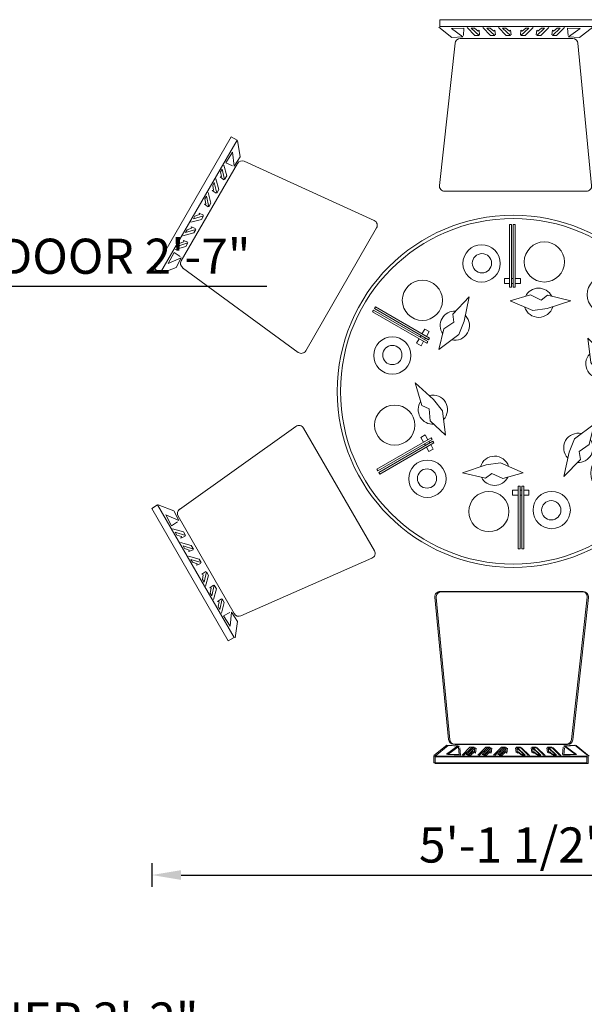
# Model space of a CAD drawing. Units: inches. Extents: x 1961 to 3038, y 800 to 1438.
# Tile 5 of 13: x 2755 to 2803, y 1058 to 1143. Entities that reach past the tile are written whole.
import ezdxf

# ---------------------------------------------------------------- set-up
doc = ezdxf.new("R2010")
doc.units = ezdxf.units.IN
doc.layers.add('A-ANNO-DIMS', color=2, linetype='Continuous', lineweight=18)
doc.layers.add('A-FURN', color=8, linetype='Continuous', lineweight=18)
doc.styles.get("Standard").update_dxf_attribs({"font": 'arial.ttf'})
doc.dimstyles.new('ISO-25', dxfattribs={"dimtxt": 3, "dimasz": 2.5, "dimexe": 1, "dimexo": 1, "dimtad": 1, "dimdec": 4, "dimlunit": 4, "dimtxsty": 'Standard', "dimcen": 2.5, "dimadec": 0, "dimazin": 0, "dimtfac": 1, "dimtdec": 4, "dimtmove": 0, "dimatfit": 3, "dimfxl": 1, "dimfxlon": 1, "dimarcsym": 0})

# ---------------------------------------------------------------- blocks, each defined once
blk = doc.blocks.new('A$C1C317F9A')
for p, q in [((0.8788, 2.2685), (0.8788, 2.2478)), ((1.3449, 2.2685), (0.8788, 2.2685)), ((1.3449, 2.2478), (1.3449, 2.2685)), ((0.8756, 2.2462), (0.9155, 2.2143)), ((0.8788, 2.2478), (1.3449, 2.2478)), ((0.9139, 2.2414), (0.9522, 2.243)), ((0.949, 2.2159), (0.9139, 2.2414)), ((0.9522, 2.243), (0.9506, 2.2206)), ((0.9618, 2.2446), (0.9857, 2.2206)), ((0.9745, 2.243), (0.9841, 2.243)), ((0.9985, 2.2206), (0.9745, 2.243)), ((0.9841, 2.243), (0.9953, 2.2334)), ((0.9953, 2.2334), (0.9985, 2.2366)), ((0.9985, 2.2366), (1.0001, 2.2222)), ((1.0097, 2.2446), (1.0336, 2.2206)), ((1.0224, 2.243), (1.032, 2.243)), ((1.0464, 2.2206), (1.0224, 2.243)), ((1.032, 2.243), (1.0432, 2.2334)), ((1.0432, 2.2334), (1.0464, 2.2366)), ((1.0464, 2.2366), (1.048, 2.2222)), ((1.0576, 2.2446), (1.0815, 2.2206)), ((1.0703, 2.243), (1.0799, 2.243)), ((1.0943, 2.2206), (1.0703, 2.243)), ((1.0799, 2.243), (1.0911, 2.2334)), ((1.0911, 2.2334), (1.0943, 2.2366)), ((1.0943, 2.2366), (1.0959, 2.2222)), ((1.1262, 2.2366), (1.1246, 2.2222)), ((1.1262, 2.2206), (1.1502, 2.243)), ((1.1294, 2.2334), (1.1262, 2.2366)), ((1.1406, 2.243), (1.1294, 2.2334)), ((1.1629, 2.2446), (1.139, 2.2206)), ((1.1502, 2.243), (1.1406, 2.243)), ((1.1741, 2.2366), (1.1725, 2.2222)), ((1.1741, 2.2206), (1.1981, 2.243)), ((1.1773, 2.2334), (1.1741, 2.2366)), ((1.1885, 2.243), (1.1773, 2.2334)), ((1.2108, 2.2446), (1.1869, 2.2206)), ((1.1981, 2.243), (1.1885, 2.243)), ((1.222, 2.2366), (1.2204, 2.2222)), ((1.222, 2.2206), (1.246, 2.243)), ((1.2252, 2.2334), (1.222, 2.2366)), ((1.2364, 2.243), (1.2252, 2.2334)), ((1.2587, 2.2446), (1.2348, 2.2206)), ((1.246, 2.243), (1.2364, 2.243)), ((1.2683, 2.243), (1.2699, 2.2206)), ((1.3066, 2.2414), (1.2683, 2.243)), ((1.2715, 2.2159), (1.3066, 2.2414)), ((1.3449, 2.2462), (1.305, 2.2143)), ((0.8775, 1.7628), (0.9251, 2.1968)), ((0.9155, 2.2143), (0.949, 2.2159)), ((0.941, 2.2111), (1.2841, 2.2111)), ((0.9857, 2.2206), (0.9985, 2.2206)), ((1.0336, 2.2206), (1.0464, 2.2206)), ((1.0815, 2.2206), (1.0943, 2.2206)), ((1.139, 2.2206), (1.1262, 2.2206)), ((1.1869, 2.2206), (1.1741, 2.2206)), ((1.2348, 2.2206), (1.222, 2.2206)), ((1.305, 2.2143), (1.2715, 2.2159)), ((1.3, 2.1966), (1.3417, 1.7626)), ((0.2422, 1.9115), (0.0091, 1.5078)), ((0.0271, 1.4974), (0.2602, 1.9011)), ((0.2602, 1.9011), (0.2422, 1.9115)), ((0.2615, 1.9003), (0.2692, 1.8498)), ((1.9724, 1.8957), (1.9544, 1.8854)), ((2.2055, 1.492), (1.9724, 1.8957)), ((0.2465, 1.8648), (0.226, 1.8324)), ((0.2511, 1.8216), (0.2465, 1.8648)), ((1.9514, 1.8873), (1.9438, 1.8368)), ((1.9544, 1.8854), (2.1875, 1.4816)), ((0.226, 1.8324), (0.2461, 1.8226)), ((0.2692, 1.8498), (0.2511, 1.8216)), ((0.282, 1.8367), (0.6787, 1.6557)), ((1.9438, 1.8368), (1.9619, 1.8086)), ((1.9619, 1.8086), (1.9665, 1.8518)), ((1.9665, 1.8518), (1.987, 1.8194)), ((0.09, 1.5329), (0.2615, 1.8301)), ((0.2148, 1.813), (0.21, 1.8047)), ((0.21, 1.8047), (0.2127, 1.7903)), ((0.2222, 1.7811), (0.2148, 1.813)), ((0.2198, 1.8249), (0.2286, 1.7922)), ((1.5338, 1.644), (1.9335, 1.8198)), ((1.9537, 1.8131), (2.1253, 1.516)), ((1.987, 1.8194), (1.9669, 1.8096)), ((1.9932, 1.8119), (1.9844, 1.7792)), ((0.1959, 1.7834), (0.2046, 1.7507)), ((0.2127, 1.7903), (0.2084, 1.7891)), ((0.2084, 1.7891), (0.22, 1.7805)), ((0.2286, 1.7922), (0.2222, 1.7811)), ((1.9844, 1.7792), (1.9908, 1.7681)), ((1.9908, 1.7681), (1.9982, 1.8)), ((2.0046, 1.7761), (1.993, 1.7675)), ((1.9982, 1.8), (2.003, 1.7917)), ((2.003, 1.7917), (2.0003, 1.7773)), ((2.0003, 1.7773), (2.0046, 1.7761)), ((0.1719, 1.7419), (0.1807, 1.7092)), ((0.1888, 1.7488), (0.1844, 1.7476)), ((0.1844, 1.7476), (0.1961, 1.7391)), ((0.1909, 1.7716), (0.1861, 1.7633)), ((0.1861, 1.7633), (0.1888, 1.7488)), ((0.1982, 1.7396), (0.1909, 1.7716)), ((0.2046, 1.7507), (0.1982, 1.7396)), ((1.3258, 1.7451), (0.8934, 1.7451)), ((2.0171, 1.7704), (2.0084, 1.7377)), ((2.0147, 1.7266), (2.0221, 1.7585)), ((2.0221, 1.7585), (2.0269, 1.7502)), ((2.0269, 1.7502), (2.0242, 1.7358)), ((0.1669, 1.7301), (0.1621, 1.7218)), ((0.1621, 1.7218), (0.1648, 1.7073)), ((0.1743, 1.6982), (0.1669, 1.7301)), ((2.0084, 1.7377), (2.0147, 1.7266)), ((2.0286, 1.7346), (2.0169, 1.726)), ((2.0242, 1.7358), (2.0286, 1.7346)), ((2.0411, 1.7289), (2.0323, 1.6962)), ((2.0387, 1.6852), (2.0461, 1.7171)), ((2.0461, 1.7171), (2.0509, 1.7088)), ((0.1648, 1.7073), (0.1605, 1.7061)), ((0.1605, 1.7061), (0.1721, 1.6976)), ((0.1807, 1.7092), (0.1743, 1.6982)), ((2.0323, 1.6962), (2.0387, 1.6852)), ((2.0525, 1.6931), (2.0409, 1.6846)), ((2.0509, 1.7088), (2.0482, 1.6943)), ((2.0482, 1.6943), (2.0525, 1.6931)), ((0.1192, 1.6507), (0.1519, 1.6595)), ((0.1583, 1.6705), (0.127, 1.6609)), ((0.127, 1.6609), (0.1318, 1.6692)), ((0.1318, 1.6692), (0.1457, 1.6741)), ((0.1445, 1.6785), (0.1577, 1.6727)), ((0.1457, 1.6741), (0.1445, 1.6785)), ((0.1519, 1.6595), (0.1583, 1.6705)), ((2.0547, 1.6575), (2.086, 1.6479)), ((2.061, 1.6464), (2.0547, 1.6575)), ((2.0685, 1.6655), (2.0552, 1.6597)), ((2.0673, 1.6611), (2.0685, 1.6655)), ((2.0812, 1.6562), (2.0673, 1.6611)), ((2.086, 1.6479), (2.0812, 1.6562)), ((0.1344, 1.629), (0.1031, 1.6195)), ((0.1031, 1.6195), (0.1078, 1.6278)), ((0.1078, 1.6278), (0.1217, 1.6327)), ((0.1217, 1.6327), (0.1206, 1.637)), ((0.1206, 1.637), (0.1338, 1.6312)), ((0.128, 1.618), (0.1344, 1.629)), ((0.6859, 1.6332), (0.4697, 1.2588)), ((1.091, 1.6437, 0.0908), (1.091, 1.4528, 0.0908)), ((1.097, 1.6437, 0.0908), (1.091, 1.6437, 0.0908)), ((1.097, 1.4528, 0.0908), (1.097, 1.6437, 0.0908)), ((1.1023, 1.6437, 0.0908), (1.1023, 1.4528, 0.0908)), ((1.1083, 1.6437, 0.0908), (1.1023, 1.6437, 0.0908)), ((1.1083, 1.4528, 0.0908), (1.1083, 1.6437, 0.0908)), ((2.0937, 1.6377), (2.061, 1.6464)), ((2.0924, 1.624), (2.0792, 1.6182)), ((2.0913, 1.6196), (2.0924, 1.624)), ((0.0953, 1.6092), (0.128, 1.618)), ((0.0966, 1.5955), (0.1098, 1.5897)), ((0.0978, 1.5912), (0.0966, 1.5955)), ((1.7426, 1.2469), (1.5264, 1.6214)), ((2.0786, 1.616), (2.1099, 1.6065)), ((2.085, 1.605), (2.0786, 1.616)), ((2.1177, 1.5962), (2.085, 1.605)), ((2.1051, 1.6148), (2.0913, 1.6196)), ((2.1099, 1.6065), (2.1051, 1.6148)), ((0.0713, 1.5677), (0.104, 1.5765)), ((0.1104, 1.5876), (0.0791, 1.578)), ((0.0791, 1.578), (0.0839, 1.5863)), ((0.0839, 1.5863), (0.0978, 1.5912)), ((0.104, 1.5765), (0.1104, 1.5876)), ((2.1026, 1.5745), (2.1339, 1.565)), ((2.1089, 1.5635), (2.1026, 1.5745)), ((2.1164, 1.5825), (2.1031, 1.5767)), ((2.1416, 1.5547), (2.1089, 1.5635)), ((2.1152, 1.5782), (2.1164, 1.5825)), ((2.1291, 1.5733), (2.1152, 1.5782)), ((2.1339, 1.565), (2.1291, 1.5733)), ((0.0502, 1.5246), (0.0679, 1.5586)), ((0.0898, 1.5423), (0.0502, 1.5246)), ((0.0679, 1.5586), (0.0865, 1.5461)), ((0.0745, 1.5125), (0.0898, 1.5423)), ((2.145, 1.5456), (2.1265, 1.5331)), ((2.1628, 1.5116), (2.145, 1.5456)), ((0.0091, 1.5078), (0.0271, 1.4974)), ((0.0269, 1.4939), (0.0745, 1.5125)), ((0.4464, 1.2539), (0.0943, 1.5121)), ((2.1232, 1.5293), (2.1628, 1.5116)), ((2.1385, 1.4995), (2.1232, 1.5293)), ((1.0755, 1.4796, 0.0908), (1.0755, 1.4641, 0.0908)), ((1.091, 1.4796, 0.0908), (1.0755, 1.4796, 0.0908)), ((1.1023, 1.4796, 0.0908), (1.097, 1.4796, 0.0908)), ((1.125, 1.4796, 0.0908), (1.1083, 1.4796, 0.0908)), ((1.125, 1.4641, 0.0908), (1.125, 1.4796, 0.0908)), ((2.1208, 1.495), (1.7657, 1.2419)), ((2.1861, 1.4809), (2.1385, 1.4995)), ((2.1875, 1.4816), (2.2055, 1.492)), ((1.0755, 1.4641, 0.0908), (1.091, 1.4641, 0.0908)), ((1.091, 1.4528, 0.0908), (1.097, 1.4528, 0.0908)), ((1.097, 1.4641, 0.0908), (1.1023, 1.4641, 0.0908)), ((1.1023, 1.4528, 0.0908), (1.1083, 1.4528, 0.0908)), ((1.1083, 1.4641, 0.0908), (1.125, 1.4641, 0.0908)), ((0.9684, 1.4231, 0.0908), (0.9184, 1.3706, 0.0908)), ((0.953, 1.3489, 0.0908), (0.9684, 1.4231, 0.0908)), ((1.1549, 1.429, 0.0908), (1.0933, 1.4112, 0.0908)), ((1.1882, 1.4134, 0.0908), (1.1549, 1.429, 0.0908)), ((1.2075, 1.4282, 0.0908), (1.1882, 1.4134, 0.0908)), ((1.278, 1.4112, 0.0908), (1.2075, 1.4282, 0.0908)), ((1.5304, 1.4154, 0.0908), (1.365, 1.3199, 0.0908)), ((1.5334, 1.4102, 0.0908), (1.5304, 1.4154, 0.0908)), ((0.6765, 1.3825, 0.0908), (0.6735, 1.3774, 0.0908)), ((0.8419, 1.2871, 0.0908), (0.6765, 1.3825, 0.0908)), ((0.6822, 1.3924, 0.0908), (0.6792, 1.3872, 0.0908)), ((0.6792, 1.3872, 0.0908), (0.8446, 1.2917, 0.0908)), ((0.8476, 1.2969, 0.0908), (0.6822, 1.3924, 0.0908)), ((1.0933, 1.4112, 0.0908), (1.1623, 1.3815, 0.0908)), ((1.1623, 1.3815, 0.0908), (1.2061, 1.3874, 0.0908)), ((1.2061, 1.3874, 0.0908), (1.278, 1.4112, 0.0908)), ((1.368, 1.3147, 0.0908), (1.5334, 1.4102, 0.0908)), ((1.5361, 1.4055, 0.0908), (1.3707, 1.3101, 0.0908)), ((1.3737, 1.3049, 0.0908), (1.539, 1.4004, 0.0908)), ((1.539, 1.4004, 0.0908), (1.5361, 1.4055, 0.0908)), ((0.6735, 1.3774, 0.0908), (0.8389, 1.2819, 0.0908)), ((0.9184, 1.3706, 0.0908), (0.9216, 1.3464, 0.0908)), ((0.8327, 1.3248, 0.0908), (0.8243, 1.3103, 0.0908)), ((0.8461, 1.317, 0.0908), (0.8327, 1.3248, 0.0908)), ((0.8914, 1.3253, 0.0908), (0.8761, 1.2631, 0.0908)), ((0.9216, 1.3464, 0.0908), (0.8914, 1.3253, 0.0908)), ((0.9363, 1.308, 0.0908), (0.953, 1.3489, 0.0908)), ((1.3805, 1.3467, 0.0908), (1.3671, 1.339, 0.0908)), ((1.3671, 1.339, 0.0908), (1.3748, 1.3255, 0.0908)), ((1.3883, 1.3333, 0.0908), (1.3805, 1.3467, 0.0908)), ((1.3939, 1.3235, 0.0908), (1.3912, 1.3281, 0.0908)), ((0.8156, 1.2953, 0.0908), (0.8079, 1.2819, 0.0908)), ((0.8213, 1.3051, 0.0908), (0.8186, 1.3005, 0.0908)), ((0.8321, 1.2927, 0.0908), (0.8348, 1.2974, 0.0908)), ((0.8377, 1.3025, 0.0908), (0.8461, 1.317, 0.0908)), ((0.8446, 1.2917, 0.0908), (0.8476, 1.2969, 0.0908)), ((0.8761, 1.2631, 0.0908), (0.9363, 1.308, 0.0908)), ((1.3763, 1.2527, 0.0908), (1.3301, 1.2971, 0.0908)), ((1.3301, 1.2971, 0.0908), (1.3389, 1.2225, 0.0908)), ((1.365, 1.3199, 0.0908), (1.368, 1.3147, 0.0908)), ((1.3707, 1.3101, 0.0908), (1.3737, 1.3049, 0.0908)), ((1.3778, 1.3204, 0.0908), (1.3805, 1.3157, 0.0908)), ((1.3835, 1.3106, 0.0908), (1.3918, 1.2961, 0.0908)), ((1.3918, 1.2961, 0.0908), (1.4053, 1.3038, 0.0908)), ((1.4053, 1.3038, 0.0908), (1.3969, 1.3183, 0.0908)), ((0.8079, 1.2819, 0.0908), (0.8213, 1.2741, 0.0908)), ((0.8213, 1.2741, 0.0908), (0.8291, 1.2876, 0.0908)), ((0.8389, 1.2819, 0.0908), (0.8419, 1.2871, 0.0908)), ((1.3795, 1.216, 0.0908), (1.3763, 1.2527, 0.0908)), ((1.3389, 1.2225, 0.0908), (1.366, 1.1876, 0.0908)), ((1.402, 1.2067, 0.0908), (1.3795, 1.216, 0.0908)), ((1.4225, 1.1371, 0.0908), (1.402, 1.2067, 0.0908)), ((1.366, 1.1876, 0.0908), (1.4225, 1.1371, 0.0908)), ((0.8033, 1.1609, 0.0908), (0.8238, 1.0913, 0.0908)), ((0.8599, 1.1105, 0.0908), (0.8033, 1.1609, 0.0908)), ((0.8238, 1.0913, 0.0908), (0.8463, 1.0821, 0.0908)), ((0.8463, 1.0821, 0.0908), (0.8495, 1.0454, 0.0908)), ((0.8869, 1.0755, 0.0908), (0.8599, 1.1105, 0.0908)), ((0.8957, 1.0009, 0.0908), (0.8869, 1.0755, 0.0908)), ((0.0847, 0.7751), (0.4398, 1.0281)), ((0.4628, 1.0231), (0.679, 0.6486)), ((0.8495, 1.0454, 0.0908), (0.8957, 1.0009, 0.0908)), ((1.3498, 1.0349, 0.0908), (1.2896, 0.99, 0.0908)), ((1.3344, 0.9727, 0.0908), (1.3498, 1.0349, 0.0908)), ((1.4045, 1.0239, 0.0908), (1.3968, 1.0105, 0.0908)), ((1.418, 1.0162, 0.0908), (1.4045, 1.0239, 0.0908)), ((0.8522, 0.9931, 0.0908), (0.6868, 0.8977, 0.0908)), ((0.834, 1.0019, 0.0908), (0.8206, 0.9942, 0.0908)), ((0.8206, 0.9942, 0.0908), (0.8289, 0.9797, 0.0908)), ((0.8424, 0.9875, 0.0908), (0.834, 1.0019, 0.0908)), ((0.8552, 0.988, 0.0908), (0.8522, 0.9931, 0.0908)), ((1.3813, 1.0063, 0.0908), (1.3783, 1.0011, 0.0908)), ((1.3783, 1.0011, 0.0908), (1.5437, 0.9057, 0.0908)), ((1.3881, 0.9955, 0.0908), (1.3797, 0.981, 0.0908)), ((1.5466, 0.9108, 0.0908), (1.3813, 1.0063, 0.0908)), ((1.3869, 1.0161, 0.0908), (1.384, 1.011, 0.0908)), ((1.384, 1.011, 0.0908), (1.5493, 0.9155, 0.0908)), ((1.5523, 0.9207, 0.0908), (1.3869, 1.0161, 0.0908)), ((1.3938, 1.0053, 0.0908), (1.3911, 1.0006, 0.0908)), ((1.4045, 0.9929, 0.0908), (1.4072, 0.9975, 0.0908)), ((1.4102, 1.0027, 0.0908), (1.418, 1.0162, 0.0908)), ((1.5196, 0.6368), (1.7358, 1.0113)), ((1.7591, 1.0162), (2.1111, 0.7579)), ((0.6898, 0.8925, 0.0908), (0.8552, 0.988, 0.0908)), ((0.8578, 0.9833, 0.0908), (0.6925, 0.8878, 0.0908)), ((0.6955, 0.8827, 0.0908), (0.8608, 0.9781, 0.0908)), ((0.8319, 0.9745, 0.0908), (0.8346, 0.9699, 0.0908)), ((0.8376, 0.9647, 0.0908), (0.8453, 0.9513, 0.0908)), ((0.848, 0.9776, 0.0908), (0.8453, 0.9823, 0.0908)), ((0.8588, 0.959, 0.0908), (0.851, 0.9725, 0.0908)), ((0.8608, 0.9781, 0.0908), (0.8578, 0.9833, 0.0908)), ((1.2896, 0.99, 0.0908), (1.2728, 0.9491, 0.0908)), ((1.3042, 0.9516, 0.0908), (1.3344, 0.9727, 0.0908)), ((1.3797, 0.981, 0.0908), (1.3932, 0.9732, 0.0908)), ((1.3932, 0.9732, 0.0908), (1.4015, 0.9877, 0.0908)), ((0.8453, 0.9513, 0.0908), (0.8588, 0.959, 0.0908)), ((1.2728, 0.9491, 0.0908), (1.2574, 0.875, 0.0908)), ((1.3074, 0.9275, 0.0908), (1.3042, 0.9516, 0.0908)), ((1.0198, 0.9106, 0.0908), (0.9478, 0.8869, 0.0908)), ((1.0636, 0.9165, 0.0908), (1.0198, 0.9106, 0.0908)), ((1.1326, 0.8869, 0.0908), (1.0636, 0.9165, 0.0908)), ((1.2574, 0.875, 0.0908), (1.3074, 0.9275, 0.0908)), ((1.5437, 0.9057, 0.0908), (1.5466, 0.9108, 0.0908)), ((1.5493, 0.9155, 0.0908), (1.5523, 0.9207, 0.0908)), ((0.6868, 0.8977, 0.0908), (0.6898, 0.8925, 0.0908)), ((0.6925, 0.8878, 0.0908), (0.6955, 0.8827, 0.0908)), ((0.9478, 0.8869, 0.0908), (1.0183, 0.8698, 0.0908)), ((1.0183, 0.8698, 0.0908), (1.0376, 0.8846, 0.0908)), ((1.0376, 0.8846, 0.0908), (1.071, 0.8691, 0.0908)), ((1.071, 0.8691, 0.0908), (1.1326, 0.8869, 0.0908)), ((1.1235, 0.8453, 0.0908), (1.1175, 0.8453, 0.0908)), ((1.1175, 0.8453, 0.0908), (1.1175, 0.6543, 0.0908)), ((1.1235, 0.6543, 0.0908), (1.1235, 0.8453, 0.0908)), ((1.1349, 0.8453, 0.0908), (1.1289, 0.8453, 0.0908)), ((1.1289, 0.8453, 0.0908), (1.1289, 0.6543, 0.0908)), ((1.1349, 0.6543, 0.0908), (1.1349, 0.8453, 0.0908)), ((1.1175, 0.8339, 0.0908), (1.1008, 0.8339, 0.0908)), ((1.1008, 0.8339, 0.0908), (1.1008, 0.8184, 0.0908)), ((1.1008, 0.8184, 0.0908), (1.1175, 0.8184, 0.0908)), ((1.1289, 0.8339, 0.0908), (1.1235, 0.8339, 0.0908)), ((1.1235, 0.8184, 0.0908), (1.1289, 0.8184, 0.0908)), ((1.1504, 0.8339, 0.0908), (1.1349, 0.8339, 0.0908)), ((1.1349, 0.8184, 0.0908), (1.1504, 0.8184, 0.0908)), ((1.1504, 0.8184, 0.0908), (1.1504, 0.8339, 0.0908)), ((0.018, 0.7884), (0, 0.778)), ((0.2511, 0.3847), (0.018, 0.7884)), ((0.0193, 0.7892), (0.0669, 0.7706)), ((0, 0.778), (0.2331, 0.3743)), ((0.0427, 0.7584), (0.0604, 0.7244)), ((0.0823, 0.7407), (0.0427, 0.7584)), ((0.0669, 0.7706), (0.0823, 0.7407)), ((0.2517, 0.4569), (0.0802, 0.7541)), ((2.1784, 0.7726), (1.9453, 0.3689)), ((1.9633, 0.3585), (2.1964, 0.7622)), ((2.131, 0.7576), (2.1156, 0.7277)), ((2.1786, 0.7762), (2.131, 0.7576)), ((2.1964, 0.7622), (2.1784, 0.7726)), ((0.0604, 0.7244), (0.079, 0.737)), ((2.1155, 0.7371), (1.9439, 0.4399)), ((2.1156, 0.7277), (2.1553, 0.7454)), ((2.1375, 0.7114), (2.119, 0.724)), ((2.1553, 0.7454), (2.1375, 0.7114)), ((0.0638, 0.7153), (0.0965, 0.7066)), ((0.0716, 0.7051), (0.0764, 0.6968)), ((0.1029, 0.6955), (0.0716, 0.7051)), ((0.0764, 0.6968), (0.0903, 0.6919)), ((0.0891, 0.6875), (0.1023, 0.6933)), ((0.0903, 0.6919), (0.0891, 0.6875)), ((0.0965, 0.7066), (0.1029, 0.6955)), ((2.1014, 0.6935), (2.095, 0.6825)), ((2.095, 0.6825), (2.1264, 0.6921)), ((2.1341, 0.7023), (2.1014, 0.6935)), ((2.1264, 0.6921), (2.1216, 0.6838)), ((0.0878, 0.6738), (0.1205, 0.6651)), ((0.0955, 0.6636), (0.1003, 0.6553)), ((0.1269, 0.654), (0.0955, 0.6636)), ((0.1205, 0.6651), (0.1269, 0.654)), ((2.1102, 0.6608), (2.0775, 0.6521)), ((2.1089, 0.6745), (2.0956, 0.6803)), ((2.1216, 0.6838), (2.1077, 0.6789)), ((2.1077, 0.6789), (2.1089, 0.6745)), ((0.1003, 0.6553), (0.1142, 0.6504)), ((0.1117, 0.6324), (0.1444, 0.6236)), ((0.1131, 0.646), (0.1263, 0.6518)), ((0.1142, 0.6504), (0.1131, 0.646)), ((1.1175, 0.6543, 0.0908), (1.1235, 0.6543, 0.0908)), ((1.1289, 0.6543, 0.0908), (1.1349, 0.6543, 0.0908)), ((2.0775, 0.6521), (2.0711, 0.641)), ((2.0711, 0.641), (2.1024, 0.6506)), ((2.0849, 0.633), (2.0717, 0.6388)), ((2.0976, 0.6423), (2.0837, 0.6374)), ((2.0837, 0.6374), (2.0849, 0.633)), ((2.1024, 0.6506), (2.0976, 0.6423)), ((0.1195, 0.6221), (0.1243, 0.6138)), ((0.1508, 0.6125), (0.1195, 0.6221)), ((0.1243, 0.6138), (0.1382, 0.6089)), ((0.137, 0.6046), (0.1502, 0.6104)), ((0.1382, 0.6089), (0.137, 0.6046)), ((0.1444, 0.6236), (0.1508, 0.6125)), ((0.6716, 0.6261), (0.272, 0.4503)), ((1.9235, 0.4334), (1.5268, 0.6143)), ((2.0535, 0.6106), (2.0471, 0.5995)), ((2.0471, 0.5995), (2.0785, 0.6091)), ((2.0862, 0.6194), (2.0535, 0.6106)), ((2.0737, 0.6008), (2.0598, 0.5959)), ((2.0785, 0.6091), (2.0737, 0.6008)), ((0.153, 0.5769), (0.1646, 0.5855)), ((0.1573, 0.5757), (0.153, 0.5769)), ((0.1546, 0.5613), (0.1573, 0.5757)), ((0.1668, 0.5849), (0.1594, 0.553)), ((0.1644, 0.5411), (0.1732, 0.5738)), ((0.1732, 0.5738), (0.1668, 0.5849)), ((2.0248, 0.5608), (2.0312, 0.5719)), ((2.0312, 0.5719), (2.0386, 0.54)), ((2.045, 0.5639), (2.0334, 0.5725)), ((2.061, 0.5915), (2.0477, 0.5973)), ((2.0598, 0.5959), (2.061, 0.5915)), ((0.1594, 0.553), (0.1546, 0.5613)), ((0.1769, 0.5354), (0.1885, 0.544)), ((0.1907, 0.5434), (0.1834, 0.5115)), ((0.1971, 0.5323), (0.1907, 0.5434)), ((2.0336, 0.5281), (2.0248, 0.5608)), ((2.0386, 0.54), (2.0433, 0.5483)), ((2.0406, 0.5627), (2.045, 0.5639)), ((2.0433, 0.5483), (2.0406, 0.5627)), ((0.1813, 0.5343), (0.1769, 0.5354)), ((0.1786, 0.5198), (0.1813, 0.5343)), ((0.1834, 0.5115), (0.1786, 0.5198)), ((0.1884, 0.4996), (0.1971, 0.5323)), ((0.8797, 0.5249), (1.3121, 0.5249)), ((0.8838, 0.5234), (1.3162, 0.5234)), ((2.0009, 0.5193), (2.0072, 0.5304)), ((2.0096, 0.4866), (2.0009, 0.5193)), ((2.0072, 0.5304), (2.0146, 0.4985)), ((2.0211, 0.5224), (2.0094, 0.531)), ((2.0167, 0.5212), (2.0211, 0.5224)), ((2.0194, 0.5068), (2.0167, 0.5212)), ((0.2009, 0.4939), (0.2125, 0.5025)), ((0.2052, 0.4928), (0.2009, 0.4939)), ((0.2025, 0.4783), (0.2052, 0.4928)), ((0.2147, 0.5019), (0.2073, 0.47)), ((0.2123, 0.4582), (0.2211, 0.4909)), ((0.2211, 0.4909), (0.2147, 0.5019)), ((0.9055, 0.0734), (0.8638, 0.5074)), ((0.9096, 0.0719), (0.8679, 0.5059)), ((1.328, 0.5072), (1.2804, 0.0732)), ((1.3321, 0.5057), (1.2845, 0.0717)), ((1.9769, 0.4779), (1.9833, 0.4889)), ((1.9833, 0.4889), (1.9907, 0.457)), ((1.9971, 0.4809), (1.9855, 0.4895)), ((1.9927, 0.4798), (1.9971, 0.4809)), ((2.0146, 0.4985), (2.0194, 0.5068)), ((0.2073, 0.47), (0.2025, 0.4783)), ((0.2185, 0.4507), (0.2386, 0.4604)), ((0.239, 0.4183), (0.2185, 0.4507)), ((0.2436, 0.4615), (0.239, 0.4183)), ((0.2617, 0.4332), (0.2436, 0.4615)), ((1.9857, 0.4451), (1.9769, 0.4779)), ((1.9907, 0.457), (1.9955, 0.4653)), ((1.9955, 0.4653), (1.9927, 0.4798)), ((0.254, 0.3827), (0.2617, 0.4332)), ((1.9363, 0.4202), (1.9544, 0.4484)), ((1.9544, 0.4484), (1.9589, 0.4053)), ((1.9589, 0.4053), (1.9795, 0.4377)), ((1.9795, 0.4377), (1.9593, 0.4474)), ((1.9439, 0.3697), (1.9363, 0.4202)), ((0.2331, 0.3743), (0.2511, 0.3847)), ((1.9453, 0.3689), (1.9633, 0.3585)), ((0.8605, 0.0239), (0.9005, 0.0558)), ((0.8647, 0.0223), (0.9046, 0.0543)), ((0.934, 0.0542), (0.8989, 0.0286)), ((0.9005, 0.0558), (0.934, 0.0542)), ((0.9381, 0.0527), (0.903, 0.0271)), ((0.9046, 0.0543), (0.9381, 0.0527)), ((1.2645, 0.059), (0.9213, 0.059)), ((1.2686, 0.0574), (0.9255, 0.0574)), ((0.9372, 0.027), (0.9356, 0.0494)), ((0.9413, 0.0255), (0.9397, 0.0479)), ((0.9468, 0.0255), (0.9707, 0.0494)), ((0.9509, 0.0239), (0.9748, 0.0479)), ((0.9835, 0.0494), (0.9595, 0.027)), ((0.9876, 0.0479), (0.9636, 0.0255)), ((0.9691, 0.027), (0.9803, 0.0366)), ((0.9707, 0.0494), (0.9835, 0.0494)), ((0.9732, 0.0255), (0.9844, 0.0351)), ((0.9748, 0.0479), (0.9876, 0.0479)), ((0.9803, 0.0366), (0.9835, 0.0334)), ((0.9835, 0.0334), (0.9851, 0.0478)), ((0.9844, 0.0351), (0.9876, 0.0319)), ((0.9876, 0.0319), (0.9892, 0.0463)), ((0.9946, 0.0255), (1.0186, 0.0494)), ((0.9988, 0.0239), (1.0227, 0.0479)), ((1.0314, 0.0494), (1.0074, 0.027)), ((1.0355, 0.0479), (1.0115, 0.0255)), ((1.017, 0.027), (1.0282, 0.0366)), ((1.0186, 0.0494), (1.0314, 0.0494)), ((1.0211, 0.0255), (1.0323, 0.0351)), ((1.0227, 0.0479), (1.0355, 0.0479)), ((1.0282, 0.0366), (1.0314, 0.0334)), ((1.0314, 0.0334), (1.033, 0.0478)), ((1.0323, 0.0351), (1.0355, 0.0319)), ((1.0355, 0.0319), (1.0371, 0.0463)), ((1.0425, 0.0255), (1.0665, 0.0494)), ((1.0467, 0.0239), (1.0706, 0.0479)), ((1.0793, 0.0494), (1.0553, 0.027)), ((1.0834, 0.0479), (1.0594, 0.0255)), ((1.0649, 0.027), (1.0761, 0.0366)), ((1.0665, 0.0494), (1.0793, 0.0494)), ((1.069, 0.0255), (1.0802, 0.0351)), ((1.0706, 0.0479), (1.0834, 0.0479)), ((1.0761, 0.0366), (1.0793, 0.0334)), ((1.0793, 0.0334), (1.0809, 0.0478)), ((1.0802, 0.0351), (1.0834, 0.0319)), ((1.0834, 0.0319), (1.085, 0.0463)), ((1.1112, 0.0334), (1.1096, 0.0478)), ((1.1112, 0.0494), (1.1351, 0.027)), ((1.124, 0.0494), (1.1112, 0.0494)), ((1.1144, 0.0366), (1.1112, 0.0334)), ((1.1153, 0.0319), (1.1137, 0.0463)), ((1.1256, 0.027), (1.1144, 0.0366)), ((1.1153, 0.0479), (1.1393, 0.0255)), ((1.1281, 0.0479), (1.1153, 0.0479)), ((1.1185, 0.0351), (1.1153, 0.0319)), ((1.1297, 0.0255), (1.1185, 0.0351)), ((1.1479, 0.0255), (1.124, 0.0494)), ((1.152, 0.0239), (1.1281, 0.0479)), ((1.1591, 0.0334), (1.1575, 0.0478)), ((1.1591, 0.0494), (1.183, 0.027)), ((1.1719, 0.0494), (1.1591, 0.0494)), ((1.1623, 0.0366), (1.1591, 0.0334)), ((1.1632, 0.0319), (1.1616, 0.0463)), ((1.1735, 0.027), (1.1623, 0.0366)), ((1.1632, 0.0479), (1.1872, 0.0255)), ((1.176, 0.0479), (1.1632, 0.0479)), ((1.1664, 0.0351), (1.1632, 0.0319)), ((1.1776, 0.0255), (1.1664, 0.0351)), ((1.1958, 0.0255), (1.1719, 0.0494)), ((1.1999, 0.0239), (1.176, 0.0479)), ((1.207, 0.0334), (1.2054, 0.0478)), ((1.207, 0.0494), (1.2309, 0.027)), ((1.2198, 0.0494), (1.207, 0.0494)), ((1.2102, 0.0366), (1.207, 0.0334)), ((1.2111, 0.0319), (1.2095, 0.0463)), ((1.2214, 0.027), (1.2102, 0.0366)), ((1.2111, 0.0479), (1.235, 0.0255)), ((1.2239, 0.0479), (1.2111, 0.0479)), ((1.2143, 0.0351), (1.2111, 0.0319)), ((1.2255, 0.0255), (1.2143, 0.0351)), ((1.2437, 0.0255), (1.2198, 0.0494)), ((1.2478, 0.0239), (1.2239, 0.0479)), ((1.2533, 0.027), (1.2549, 0.0494)), ((1.29, 0.0558), (1.2565, 0.0542)), ((1.2565, 0.0542), (1.2916, 0.0286)), ((1.2574, 0.0255), (1.259, 0.0479)), ((1.2941, 0.0543), (1.2606, 0.0527)), ((1.2606, 0.0527), (1.2957, 0.0271)), ((1.3299, 0.0239), (1.29, 0.0558)), ((1.334, 0.0223), (1.2941, 0.0543)), ((0.8605, 0.0223), (0.8605, 0.0015)), ((1.3267, 0.0223), (0.8605, 0.0223)), ((0.8605, 0.0015), (1.3267, 0.0015)), ((0.8647, 0.0207), (0.8647, 0)), ((1.3308, 0.0207), (0.8647, 0.0207)), ((0.8647, 0), (1.3308, 0)), ((0.8989, 0.0286), (0.9372, 0.027)), ((0.903, 0.0271), (0.9413, 0.0255)), ((0.9595, 0.027), (0.9691, 0.027)), ((0.9636, 0.0255), (0.9732, 0.0255)), ((1.0074, 0.027), (1.017, 0.027)), ((1.0115, 0.0255), (1.0211, 0.0255)), ((1.0553, 0.027), (1.0649, 0.027)), ((1.0594, 0.0255), (1.069, 0.0255)), ((1.1351, 0.027), (1.1256, 0.027)), ((1.1393, 0.0255), (1.1297, 0.0255)), ((1.183, 0.027), (1.1735, 0.027)), ((1.1872, 0.0255), (1.1776, 0.0255)), ((1.2309, 0.027), (1.2214, 0.027)), ((1.235, 0.0255), (1.2255, 0.0255)), ((1.2916, 0.0286), (1.2533, 0.027)), ((1.2957, 0.0271), (1.2574, 0.0255)), ((1.3267, 0.0015), (1.3267, 0.0223)), ((1.3308, 0), (1.3308, 0.0207))]:
    blk.add_line(p, q)
for centre, radius in [((1.1027, 1.135), 0.537), ((1.1027, 1.135), 0.527), ((1.0059, 1.525, 0.0908), 0.0569), ((1.1975, 1.5297, 0.0908), 0.0613), ((1.0072, 1.5257, 0.0908), 0.0294), ((0.8256, 1.4126, 0.0908), 0.0613), ((1.385, 1.4297, 0.0908), 0.0569), ((1.3863, 1.4289, 0.0908), 0.0294), ((1.4849, 1.2661, 0.0908), 0.0613), ((0.7338, 1.2443, 0.0908), 0.0569), ((0.7339, 1.2458, 0.0908), 0.0294), ((0.741, 1.0319, 0.0908), 0.0613), ((1.4921, 1.0537, 0.0908), 0.0569), ((1.492, 1.0522, 0.0908), 0.0294), ((1.4003, 0.8854, 0.0908), 0.0613), ((0.8408, 0.8683, 0.0908), 0.0569), ((0.8396, 0.8691, 0.0908), 0.0294), ((1.0283, 0.7683, 0.0908), 0.0613), ((1.2199, 0.773, 0.0908), 0.0569), ((1.2186, 0.7723, 0.0908), 0.0294)]:
    blk.add_circle(centre, radius)
for centre, radius, start, end in [((0.941, 2.1951), 0.016, 90, 173.7428), ((1.2841, 2.1951), 0.016, 5.4801, 90), ((0.2754, 1.8222), 0.016, 65.4801, 150), ((1.9399, 1.8052), 0.016, 30, 113.7428), ((0.8934, 1.7611), 0.016, 173.7428, 270), ((1.3258, 1.7611), 0.016, 270, 5.4801), ((0.6721, 1.6412), 0.016, 330, 65.4801), ((1.5403, 1.6294), 0.016, 113.7428, 210), ((0.1038, 1.525), 0.016, 150, 233.7428), ((2.1115, 1.508), 0.016, 305.4801, 30), ((1.1801, 1.4052, 0.0908), 0.0446, 26.6641, 154.1442), ((1.1801, 1.4052, 0.0908), 0.0446, 197.0611, 344.0662), ((0.9246, 1.3353, 0.0908), 0.0446, 86.6641, 214.1442), ((0.9246, 1.3353, 0.0908), 0.0446, 257.0611, 44.0662), ((1.3684, 1.2189, 0.0908), 0.0446, 326.6641, 94.1442), ((0.4559, 1.2667), 0.016, 233.7428, 330), ((1.3684, 1.2189, 0.0908), 0.0446, 137.0611, 284.0662), ((1.7565, 1.2549), 0.016, 210, 305.4801), ((0.8574, 1.0791, 0.0908), 0.0446, 317.0611, 104.0662), ((0.8574, 1.0791, 0.0908), 0.0446, 146.6641, 274.1442), ((0.449, 1.0151), 0.016, 30, 125.4801), ((1.3012, 0.9627, 0.0908), 0.0446, 77.0611, 224.0662), ((1.7496, 1.0033), 0.016, 53.7428, 150), ((1.3012, 0.9627, 0.0908), 0.0446, 266.6641, 34.1442), ((1.0457, 0.8928, 0.0908), 0.0446, 17.0611, 164.0662), ((1.0457, 0.8928, 0.0908), 0.0446, 206.6641, 334.1442), ((0.094, 0.7621), 0.016, 125.4801, 210), ((2.1017, 0.7451), 0.016, 330, 53.7428), ((0.6652, 0.6407), 0.016, 293.7428, 30), ((1.5334, 0.6288), 0.016, 150, 245.4801), ((0.8797, 0.5089), 0.016, 90, 185.4801), ((0.8838, 0.5074), 0.016, 90, 185.4801), ((1.3121, 0.5089), 0.016, 353.7428, 90), ((1.3162, 0.5074), 0.016, 353.7428, 90), ((0.2656, 0.4649), 0.016, 210, 293.7428), ((1.9301, 0.4479), 0.016, 245.4801, 330), ((0.9213, 0.0749), 0.016, 185.4801, 270), ((0.9255, 0.0734), 0.016, 185.4801, 270), ((1.2645, 0.0749), 0.016, 270, 353.7428), ((1.2686, 0.0734), 0.016, 270, 353.7428)]:
    blk.add_arc(centre, radius, start, end)
blk = doc.blocks.new('*D51')
at = {"layer": 'A-ANNO-DIMS', "color": 0, "lineweight": -2, "transparency": 16777216}
for p, q in [((2700.291, 1120.773), (2700.291, 1118.773)), ((2731.268, 1120.773), (2731.268, 1118.773)), ((2702.791, 1119.773), (2728.768, 1119.773)), ((2731.268, 1119.773), (2776.157, 1119.773))]:
    blk.add_line(p, q, dxfattribs=at)
at = {"layer": 'A-ANNO-DIMS', "color": 0, "transparency": 16777216}
for points in [[(2702.791, 1120.19), (2702.791, 1119.357), (2700.291, 1119.773)], [(2728.768, 1120.19), (2728.768, 1119.357), (2731.268, 1119.773)]]:
    blk.add_solid(points, dxfattribs=at)
at = {"layer": 'Defpoints', "color": 0, "transparency": 16777216}
for p in [(2700.291, 1124.42), (2731.268, 1124.42), (2731.268, 1119.773)]:
    blk.add_point(p, dxfattribs=at)
at = {"layer": 'A-ANNO-DIMS', "color": 0, "transparency": 16777216, "insert": (2754.962, 1121.95), "char_height": 3, "attachment_point": 5}
blk.add_mtext('KITCHEN DOOR 2\'-7"', dxfattribs=at)
blk = doc.blocks.new('*D62')
at = {"layer": 'A-ANNO-DIMS', "color": 0, "lineweight": -2, "transparency": 16777216}
for p, q in [((2766.339, 1070.514), (2766.339, 1068.514)), ((2828.069, 1070.514), (2828.069, 1068.514)), ((2768.839, 1069.514), (2825.569, 1069.514))]:
    blk.add_line(p, q, dxfattribs=at)
at = {"layer": 'A-ANNO-DIMS', "color": 0, "transparency": 16777216}
for points in [[(2768.839, 1069.93), (2768.839, 1069.097), (2766.339, 1069.514)], [(2825.569, 1069.93), (2825.569, 1069.097), (2828.069, 1069.514)]]:
    blk.add_solid(points, dxfattribs=at)
at = {"layer": 'Defpoints', "color": 0, "transparency": 16777216}
for p in [(2766.339, 1079.038), (2828.069, 1079.038), (2828.069, 1069.514)]:
    blk.add_point(p, dxfattribs=at)
at = {"layer": 'A-ANNO-DIMS', "color": 0, "transparency": 16777216, "insert": (2797.204, 1071.69), "char_height": 3, "attachment_point": 5}
blk.add_mtext('5\'-1 1/2"', dxfattribs=at)
blk = doc.blocks.new('*D69')
at = {"layer": 'A-ANNO-DIMS', "color": 0, "lineweight": -2, "transparency": 16777216}
for p, q in [((2687.202, 1055.563), (2687.202, 1053.563)), ((2725.322, 1055.563), (2725.322, 1053.563)), ((2689.702, 1054.563), (2722.822, 1054.563)), ((2725.322, 1054.563), (2771.964, 1054.563))]:
    blk.add_line(p, q, dxfattribs=at)
at = {"layer": 'A-ANNO-DIMS', "color": 0, "transparency": 16777216}
for points in [[(2689.702, 1054.979), (2689.702, 1054.146), (2687.202, 1054.563)], [(2722.822, 1054.979), (2722.822, 1054.146), (2725.322, 1054.563)]]:
    blk.add_solid(points, dxfattribs=at)
at = {"layer": 'Defpoints', "color": 0, "transparency": 16777216}
for p in [(2687.202, 1060.281), (2725.322, 1060.281), (2725.322, 1054.563)]:
    blk.add_point(p, dxfattribs=at)
at = {"layer": 'A-ANNO-DIMS', "color": 0, "transparency": 16777216, "insert": (2749.893, 1056.748), "char_height": 3, "attachment_point": 5}
blk.add_mtext('SINK & DRAINER 3\'-2"', dxfattribs=at)

msp = doc.modelspace()

# ---------------------------------------------------------------- block references
at = {"layer": 'A-FURN', "xscale": 27.98955775126368, "yscale": 27.98955775126368, "zscale": 27.98955775126368}
msp.add_blockref('A$C1C317F9A', (2766.339, 1079.03804, -2.54052), dxfattribs=at)

# ---------------------------------------------------------------- dimensions: what is measured, and where the dimension line sits
at = {"layer": 'A-ANNO-DIMS'}
for base, p1, p2, text, picture, middle in [((2731.26803, 1119.77324), (2700.29129, 1124.41975), (2731.26803, 1124.41975), 'KITCHEN DOOR <>', '*D51', (2754.96227, 1121.95042)), ((2725.32185, 1054.56259), (2687.20225, 1060.28053), (2725.32185, 1060.28053), 'SINK & DRAINER <>', '*D69', (2749.89296, 1056.74796))]:
    dim = msp.add_linear_dim(base=base, p1=p1, p2=p2, text=text, dimstyle='ISO-25', override={"dimdec": 1, "dimlfac": 1, "dimrnd": 0, "dimzin": 1, "dimdsep": 46, "dimlunit": 4, "dimfrac": 2}, dxfattribs=at)
    dim.commit()
    dim.dimension.update_dxf_attribs({"geometry": picture, "text_midpoint": middle})
dim = msp.add_linear_dim(base=(2828.0693, 1069.51382), p1=(2766.339, 1079.03804), p2=(2828.0693, 1079.03804), dimstyle='ISO-25', override={"dimdec": 1, "dimlfac": 1, "dimrnd": 0, "dimzin": 1, "dimdsep": 46, "dimlunit": 4, "dimfrac": 2}, dxfattribs=at)
dim.commit()
dim.dimension.update_dxf_attribs({"geometry": '*D62', "text_midpoint": (2797.20415, 1071.68998)})

doc.saveas('drawing.dxf')
